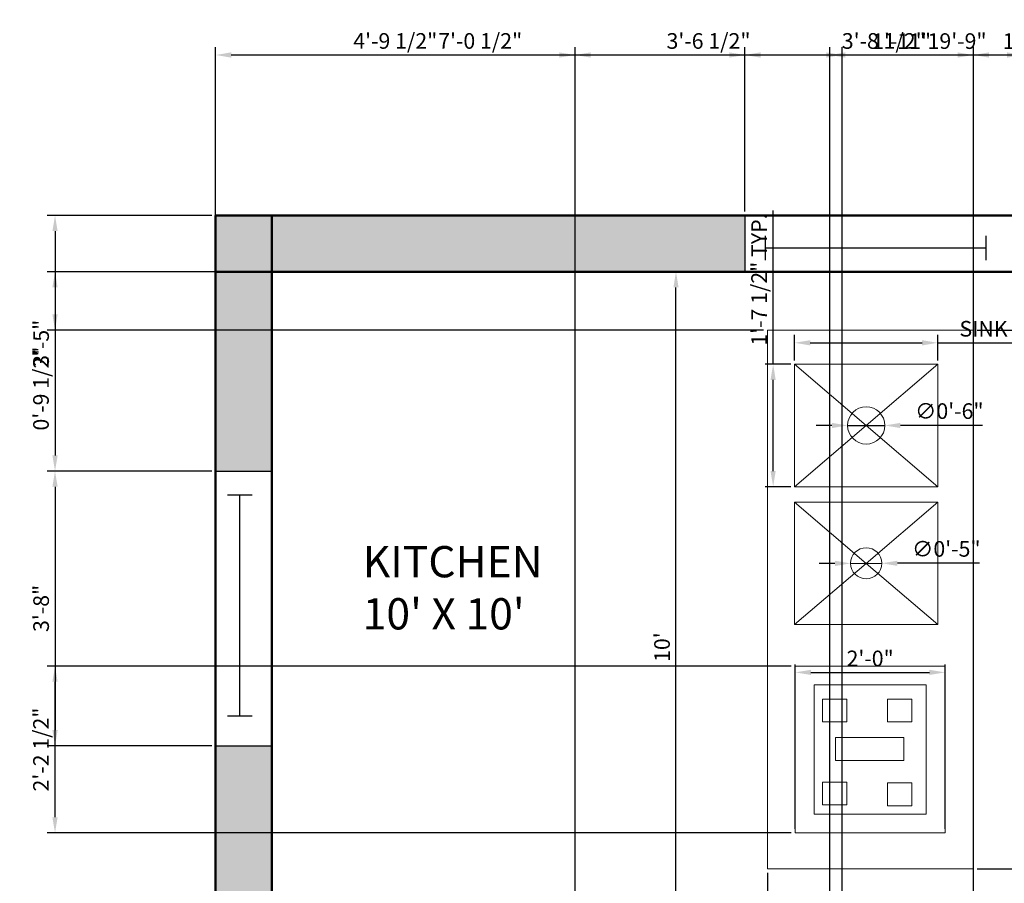
# Model space of a CAD drawing. Units: millimetres. Extents: x 2877 to 3173, y 802 to 1374.
# Tile 4 of 5: x 2877 to 3035, y 1236 to 1374. Entities that reach past the tile are written whole.
import ezdxf

# ---------------------------------------------------------------- set-up
doc = ezdxf.new("R2010")
doc.units = ezdxf.units.MM
for name, color, linetype, lineweight in [('A-AREA-IDEN', 150, 'Continuous', 25), ('A-EQPM', 70, 'Continuous', 18), ('A-FLOR-FIXT', 70, 'Continuous', 18), ('A-WALL-PATT', 3, 'Continuous', 13), ('dimensions', 140, 'Continuous', 18), ('walls', 50, 'Continuous', 50), ('windows', 190, 'Continuous', 25)]:
    doc.layers.add(name, color=color, linetype=linetype, lineweight=lineweight)
doc.styles.get("Standard").update_dxf_attribs({"font": 'arial.ttf'})
doc.dimstyles.new('ISO-25', dxfattribs={"dimtxt": 2.5, "dimasz": 2.5, "dimexe": 1.25, "dimexo": 0.625, "dimtad": 1, "dimdec": 0, "dimlunit": 3, "dimtxsty": 'Standard', "dimcen": 2.5, "dimadec": 0, "dimazin": 0, "dimtfac": 1, "dimtdec": 0, "dimtmove": 0, "dimatfit": 3, "dimfxl": 1, "dimarcsym": 0})

# ---------------------------------------------------------------- blocks, each defined once
blk = doc.blocks.new('*U4')
for p, q in [((0, 4), (0, 0)), ((36, 4), (36, 0)), ((0, 2), (36, 2))]:
    blk.add_line(p, q)
blk = doc.blocks.new('*D11')
at = {"layer": 'Defpoints', "color": 0, "transparency": 16777216}
for p in [(2982.2, 1333.28), (2982.2, 1333.28), (2982.2, 1213.28)]:
    blk.add_point(p, dxfattribs=at)
at = {"layer": 'dimensions', "color": 0, "lineweight": -2, "transparency": 16777216}
for p, q in [((2982.83, 1333.28), (2983.45, 1333.28)), ((2982.2, 1215.78), (2982.2, 1330.78)), ((2982.83, 1213.28), (2983.45, 1213.28))]:
    blk.add_line(p, q, dxfattribs=at)
at = {"layer": 'dimensions', "color": 0, "transparency": 16777216}
for points in [[(2981.79, 1330.78), (2982.62, 1330.78), (2982.2, 1333.28)], [(2981.79, 1215.78), (2982.62, 1215.78), (2982.2, 1213.28)]]:
    blk.add_solid(points, dxfattribs=at)
at = {"layer": 'dimensions', "color": 0, "transparency": 16777216, "insert": (2980.3, 1273.28), "char_height": 2.5, "attachment_point": 5, "rotation": 90}
blk.add_mtext("10'", dxfattribs=at)
blk = doc.blocks.new('SINK-BOWL')
for q in [(0, 19.57), (22.88, 19.57), (0, 0), (22.88, 0)]:
    blk.add_line((11.44, 9.78), q)
blk.add_lwpolyline([(0, 19.57), (22.88, 19.57), (22.88, 0), (0, 0)], close=True)
blk = doc.blocks.new('*D24')
at = {"layer": 'Defpoints', "color": 0, "transparency": 16777216}
for p in [(3024.04, 1321.93), (3001.16, 1318.5), (3024.04, 1318.5)]:
    blk.add_point(p, dxfattribs=at)
at = {"layer": 'dimensions', "color": 0, "lineweight": -2, "transparency": 16777216}
for p, q in [((3001.16, 1319.12), (3001.16, 1323.18)), ((3003.66, 1321.93), (3021.54, 1321.93)), ((3024.04, 1319.12), (3024.04, 1323.18)), ((3024.04, 1321.93), (3054.08, 1321.93))]:
    blk.add_line(p, q, dxfattribs=at)
at = {"layer": 'dimensions', "color": 0, "transparency": 16777216}
for points in [[(3003.66, 1322.35), (3003.66, 1321.51), (3001.16, 1321.93)], [(3021.54, 1322.35), (3021.54, 1321.51), (3024.04, 1321.93)]]:
    blk.add_solid(points, dxfattribs=at)
at = {"layer": 'dimensions', "color": 0, "transparency": 16777216, "insert": (3040.31, 1323.85), "char_height": 2.5, "attachment_point": 5}
blk.add_mtext('SINK 1\'-11" TYP.', dxfattribs=at)
blk = doc.blocks.new('*D25')
at = {"layer": 'Defpoints', "color": 0, "transparency": 16777216}
for p in [(2997.73, 1318.5), (3001.16, 1318.5), (3001.16, 1298.93)]:
    blk.add_point(p, dxfattribs=at)
at = {"layer": 'dimensions', "color": 0, "lineweight": -2, "transparency": 16777216}
for p, q in [((2997.73, 1318.5), (2997.73, 1343.08)), ((3000.53, 1318.5), (2996.48, 1318.5)), ((2997.73, 1301.43), (2997.73, 1316)), ((3000.53, 1298.93), (2996.48, 1298.93))]:
    blk.add_line(p, q, dxfattribs=at)
at = {"layer": 'dimensions', "color": 0, "transparency": 16777216}
for points in [[(2997.31, 1316), (2998.14, 1316), (2997.73, 1318.5)], [(2997.31, 1301.43), (2998.14, 1301.43), (2997.73, 1298.93)]]:
    blk.add_solid(points, dxfattribs=at)
at = {"layer": 'dimensions', "color": 0, "transparency": 16777216, "insert": (2995.81, 1332.04), "char_height": 2.5, "attachment_point": 5, "rotation": 90}
blk.add_mtext('1\'-7 1/2" TYP.', dxfattribs=at)
blk = doc.blocks.new('*D34')
at = {"layer": 'Defpoints', "color": 0, "transparency": 16777216}
for p in [(3145.62, 1367.94), (2908.62, 1342.28), (3145.62, 1342.28)]:
    blk.add_point(p, dxfattribs=at)
at = {"layer": 'dimensions', "color": 0, "lineweight": -2, "transparency": 16777216}
for p, q in [((2908.62, 1342.9), (2908.62, 1369.19)), ((3145.62, 1342.9), (3145.62, 1369.19)), ((2911.12, 1367.94), (3143.12, 1367.94))]:
    blk.add_line(p, q, dxfattribs=at)
at = {"layer": 'dimensions', "color": 0, "transparency": 16777216}
for points in [[(2911.12, 1368.36), (2911.12, 1367.52), (2908.62, 1367.94)], [(3143.12, 1368.36), (3143.12, 1367.52), (3145.62, 1367.94)]]:
    blk.add_solid(points, dxfattribs=at)
at = {"layer": 'dimensions', "color": 0, "transparency": 16777216, "insert": (3027.12, 1369.84), "char_height": 2.5, "attachment_point": 5}
blk.add_mtext('19\'-9"', dxfattribs=at)
blk = doc.blocks.new('*D36')
at = {"layer": 'Defpoints', "color": 0, "transparency": 16777216}
for p in [(2908.62, 1301.43), (2917.62, 1301.43), (2917.62, 803.61)]:
    blk.add_point(p, dxfattribs=at)
at = {"layer": 'dimensions', "color": 0, "lineweight": -2, "transparency": 16777216}
for p, q in [((2908.62, 1300.81), (2908.62, 802.36)), ((2917.62, 1300.81), (2917.62, 802.36)), ((2911.12, 803.61), (2915.12, 803.61))]:
    blk.add_line(p, q, dxfattribs=at)
at = {"layer": 'dimensions', "color": 0, "transparency": 16777216}
for points in [[(2911.12, 804.03), (2911.12, 803.2), (2908.62, 803.61)], [(2915.12, 804.03), (2915.12, 803.2), (2917.62, 803.61)]]:
    blk.add_solid(points, dxfattribs=at)
at = {"layer": 'dimensions', "color": 0, "transparency": 16777216, "insert": (2913.12, 805.52), "char_height": 2.5, "attachment_point": 5}
blk.add_mtext('0\'-9"', dxfattribs=at)
blk = doc.blocks.new('*D44')
at = {"layer": 'Defpoints', "color": 0, "transparency": 16777216}
for p in [(2996.81, 1237.82), (3029.69, 1237.82), (3029.69, 803.61)]:
    blk.add_point(p, dxfattribs=at)
at = {"layer": 'dimensions', "color": 0, "lineweight": -2, "transparency": 16777216}
for p, q in [((2996.81, 1237.19), (2996.81, 802.36)), ((3029.69, 1237.19), (3029.69, 802.36)), ((2999.31, 803.61), (3027.19, 803.61))]:
    blk.add_line(p, q, dxfattribs=at)
at = {"layer": 'dimensions', "color": 0, "transparency": 16777216}
for points in [[(2999.31, 804.03), (2999.31, 803.2), (2996.81, 803.61)], [(3027.19, 804.03), (3027.19, 803.2), (3029.69, 803.61)]]:
    blk.add_solid(points, dxfattribs=at)
at = {"layer": 'dimensions', "color": 0, "transparency": 16777216, "insert": (3013.25, 805.52), "char_height": 2.5, "attachment_point": 5}
blk.add_mtext('2\'-9"', dxfattribs=at)
blk = doc.blocks.new('*D45')
at = {"layer": 'Defpoints', "color": 0, "transparency": 16777216}
for p in [(3029.69, 1323.97), (3171.28, 1323.97), (3029.69, 1237.82)]:
    blk.add_point(p, dxfattribs=at)
at = {"layer": 'dimensions', "color": 0, "lineweight": -2, "transparency": 16777216}
for p, q in [((3030.32, 1323.97), (3172.53, 1323.97)), ((3171.28, 1240.32), (3171.28, 1321.47)), ((3030.32, 1237.82), (3172.53, 1237.82))]:
    blk.add_line(p, q, dxfattribs=at)
at = {"layer": 'dimensions', "color": 0, "transparency": 16777216}
for points in [[(3170.87, 1321.47), (3171.7, 1321.47), (3171.28, 1323.97)], [(3170.87, 1240.32), (3171.7, 1240.32), (3171.28, 1237.82)]]:
    blk.add_solid(points, dxfattribs=at)
at = {"layer": 'dimensions', "color": 0, "transparency": 16777216, "insert": (3169.4, 1280.89), "char_height": 2.5, "attachment_point": 5, "rotation": 90}
blk.add_mtext('7\'-2"', dxfattribs=at)
blk = doc.blocks.new('*D48')
at = {"layer": 'Defpoints', "color": 0, "transparency": 16777216}
for p in [(3029.73, 1367.94), (3006.77, 1144.28), (3029.73, 1144.28)]:
    blk.add_point(p, dxfattribs=at)
at = {"layer": 'dimensions', "color": 0, "lineweight": -2, "transparency": 16777216}
for p, q in [((3006.77, 1144.9), (3006.77, 1369.19)), ((3029.73, 1144.9), (3029.73, 1369.19)), ((3009.27, 1367.94), (3027.23, 1367.94))]:
    blk.add_line(p, q, dxfattribs=at)
at = {"layer": 'dimensions', "color": 0, "transparency": 16777216}
for points in [[(3009.27, 1368.36), (3009.27, 1367.52), (3006.77, 1367.94)], [(3027.23, 1368.36), (3027.23, 1367.52), (3029.73, 1367.94)]]:
    blk.add_solid(points, dxfattribs=at)
at = {"layer": 'dimensions', "color": 0, "transparency": 16777216, "insert": (3018.25, 1369.82), "char_height": 2.5, "attachment_point": 5}
blk.add_mtext('1\'-11"', dxfattribs=at)
blk = doc.blocks.new('*D49')
at = {"layer": 'Defpoints', "color": 0, "transparency": 16777216}
for p in [(3046.62, 1367.94), (3029.73, 1144.28), (3046.62, 1144.28)]:
    blk.add_point(p, dxfattribs=at)
at = {"layer": 'dimensions', "color": 0, "lineweight": -2, "transparency": 16777216}
for p, q in [((3029.73, 1144.9), (3029.73, 1369.19)), ((3046.62, 1144.9), (3046.62, 1369.19)), ((3032.23, 1367.94), (3044.12, 1367.94))]:
    blk.add_line(p, q, dxfattribs=at)
at = {"layer": 'dimensions', "color": 0, "transparency": 16777216}
for points in [[(3032.23, 1368.36), (3032.23, 1367.52), (3029.73, 1367.94)], [(3044.12, 1368.36), (3044.12, 1367.52), (3046.62, 1367.94)]]:
    blk.add_solid(points, dxfattribs=at)
at = {"layer": 'dimensions', "color": 0, "transparency": 16777216, "insert": (3038.18, 1369.84), "char_height": 2.5, "attachment_point": 5}
blk.add_mtext('1\'-5"', dxfattribs=at)
blk = doc.blocks.new('*D50')
at = {"layer": 'Defpoints', "color": 0, "transparency": 16777216}
for p in [(2908.62, 1301.43), (2882.96, 1257.52), (2908.62, 1257.52)]:
    blk.add_point(p, dxfattribs=at)
at = {"layer": 'dimensions', "color": 0, "lineweight": -2, "transparency": 16777216}
for p, q in [((2908, 1301.43), (2881.71, 1301.43)), ((2882.96, 1298.93), (2882.96, 1260.02)), ((2908, 1257.52), (2881.71, 1257.52))]:
    blk.add_line(p, q, dxfattribs=at)
at = {"layer": 'dimensions', "color": 0, "transparency": 16777216}
for points in [[(2882.54, 1298.93), (2883.38, 1298.93), (2882.96, 1301.43)], [(2882.54, 1260.02), (2883.38, 1260.02), (2882.96, 1257.52)]]:
    blk.add_solid(points, dxfattribs=at)
at = {"layer": 'dimensions', "color": 0, "transparency": 16777216, "insert": (2881.06, 1279.47), "char_height": 2.5, "attachment_point": 5, "rotation": 90}
blk.add_mtext('3\'-8"', dxfattribs=at)
blk = doc.blocks.new('*D51')
at = {"layer": 'Defpoints', "color": 0, "transparency": 16777216}
for p in [(2908.62, 1342.28), (2882.96, 1301.43), (2908.62, 1301.43)]:
    blk.add_point(p, dxfattribs=at)
at = {"layer": 'dimensions', "color": 0, "lineweight": -2, "transparency": 16777216}
for p, q in [((2908, 1342.28), (2881.71, 1342.28)), ((2882.96, 1339.78), (2882.96, 1303.93)), ((2908, 1301.43), (2881.71, 1301.43))]:
    blk.add_line(p, q, dxfattribs=at)
at = {"layer": 'dimensions', "color": 0, "transparency": 16777216}
for points in [[(2882.54, 1339.78), (2883.38, 1339.78), (2882.96, 1342.28)], [(2882.54, 1303.93), (2883.38, 1303.93), (2882.96, 1301.43)]]:
    blk.add_solid(points, dxfattribs=at)
at = {"layer": 'dimensions', "color": 0, "transparency": 16777216, "insert": (2881.06, 1321.85), "char_height": 2.5, "attachment_point": 5, "rotation": 90}
blk.add_mtext('3\'-5"', dxfattribs=at)
blk = doc.blocks.new('*D52')
at = {"layer": 'Defpoints', "color": 0, "transparency": 16777216}
for p in [(3037.62, 1367.94), (2993.21, 1342.28), (3037.62, 1342.28)]:
    blk.add_point(p, dxfattribs=at)
at = {"layer": 'dimensions', "color": 0, "lineweight": -2, "transparency": 16777216}
for p, q in [((2993.21, 1342.9), (2993.21, 1369.19)), ((3037.62, 1342.9), (3037.62, 1369.19)), ((2995.71, 1367.94), (3035.12, 1367.94))]:
    blk.add_line(p, q, dxfattribs=at)
at = {"layer": 'dimensions', "color": 0, "transparency": 16777216}
for points in [[(2995.71, 1368.36), (2995.71, 1367.52), (2993.21, 1367.94)], [(3035.12, 1368.36), (3035.12, 1367.52), (3037.62, 1367.94)]]:
    blk.add_solid(points, dxfattribs=at)
at = {"layer": 'dimensions', "color": 0, "transparency": 16777216, "insert": (3015.41, 1369.86), "char_height": 2.5, "attachment_point": 5}
blk.add_mtext('3\'-8 1/2"', dxfattribs=at)
blk = doc.blocks.new('*D53')
at = {"layer": 'Defpoints', "color": 0, "transparency": 16777216}
for p in [(2993.21, 1367.94), (2908.62, 1342.28), (2993.21, 1342.28)]:
    blk.add_point(p, dxfattribs=at)
at = {"layer": 'dimensions', "color": 0, "lineweight": -2, "transparency": 16777216}
for p, q in [((2908.62, 1342.9), (2908.62, 1369.19)), ((2993.21, 1342.9), (2993.21, 1369.19)), ((2911.12, 1367.94), (2990.71, 1367.94))]:
    blk.add_line(p, q, dxfattribs=at)
at = {"layer": 'dimensions', "color": 0, "transparency": 16777216}
for points in [[(2911.12, 1368.36), (2911.12, 1367.52), (2908.62, 1367.94)], [(2990.71, 1368.36), (2990.71, 1367.52), (2993.21, 1367.94)]]:
    blk.add_solid(points, dxfattribs=at)
at = {"layer": 'dimensions', "color": 0, "transparency": 16777216, "insert": (2950.91, 1369.86), "char_height": 2.5, "attachment_point": 5}
blk.add_mtext('7\'-0 1/2"', dxfattribs=at)
blk = doc.blocks.new('*D58')
at = {"layer": 'Defpoints', "color": 0, "transparency": 16777216}
for p in [(2966.07, 1367.94), (2908.62, 943.28), (2966.07, 943.28)]:
    blk.add_point(p, dxfattribs=at)
at = {"layer": 'dimensions', "color": 0, "lineweight": -2, "transparency": 16777216}
for p, q in [((2908.62, 943.9), (2908.62, 1369.19)), ((2966.07, 943.9), (2966.07, 1369.19)), ((2911.12, 1367.94), (2963.57, 1367.94))]:
    blk.add_line(p, q, dxfattribs=at)
at = {"layer": 'dimensions', "color": 0, "transparency": 16777216}
for points in [[(2911.12, 1368.36), (2911.12, 1367.52), (2908.62, 1367.94)], [(2963.57, 1368.36), (2963.57, 1367.52), (2966.07, 1367.94)]]:
    blk.add_solid(points, dxfattribs=at)
at = {"layer": 'dimensions', "color": 0, "transparency": 16777216, "insert": (2937.34, 1369.86), "char_height": 2.5, "attachment_point": 5}
blk.add_mtext('4\'-9 1/2"', dxfattribs=at)
blk = doc.blocks.new('*D59')
at = {"layer": 'Defpoints', "color": 0, "transparency": 16777216}
for p in [(3008.74, 1367.94), (2966.07, 943.28), (3008.74, 943.28)]:
    blk.add_point(p, dxfattribs=at)
at = {"layer": 'dimensions', "color": 0, "lineweight": -2, "transparency": 16777216}
for p, q in [((2966.07, 943.9), (2966.07, 1369.19)), ((3008.74, 943.9), (3008.74, 1369.19)), ((2968.57, 1367.94), (3006.24, 1367.94))]:
    blk.add_line(p, q, dxfattribs=at)
at = {"layer": 'dimensions', "color": 0, "transparency": 16777216}
for points in [[(2968.57, 1368.36), (2968.57, 1367.52), (2966.07, 1367.94)], [(3006.24, 1368.36), (3006.24, 1367.52), (3008.74, 1367.94)]]:
    blk.add_solid(points, dxfattribs=at)
at = {"layer": 'dimensions', "color": 0, "transparency": 16777216, "insert": (2987.4, 1369.86), "char_height": 2.5, "attachment_point": 5}
blk.add_mtext('3\'-6 1/2"', dxfattribs=at)
blk = doc.blocks.new('*D66')
at = {"layer": 'Defpoints', "color": 0, "transparency": 16777216}
for p in [(2917.62, 1257.52), (2996.81, 1237.82), (2996.81, 803.61)]:
    blk.add_point(p, dxfattribs=at)
at = {"layer": 'dimensions', "color": 0, "lineweight": -2, "transparency": 16777216}
for p, q in [((2917.62, 1256.89), (2917.62, 802.36)), ((2996.81, 1237.19), (2996.81, 802.36)), ((2920.12, 803.61), (2994.31, 803.61))]:
    blk.add_line(p, q, dxfattribs=at)
at = {"layer": 'dimensions', "color": 0, "transparency": 16777216}
for points in [[(2920.12, 804.03), (2920.12, 803.2), (2917.62, 803.61)], [(2994.31, 804.03), (2994.31, 803.2), (2996.81, 803.61)]]:
    blk.add_solid(points, dxfattribs=at)
at = {"layer": 'dimensions', "color": 0, "transparency": 16777216, "insert": (2957.22, 805.52), "char_height": 2.5, "attachment_point": 5}
blk.add_mtext('6\'-7"', dxfattribs=at)
blk = doc.blocks.new('*D67')
at = {"layer": 'Defpoints', "color": 0, "transparency": 16777216}
for p in [(2993.21, 1333.28), (2882.96, 1323.97), (2996.81, 1323.97)]:
    blk.add_point(p, dxfattribs=at)
at = {"layer": 'dimensions', "color": 0, "lineweight": -2, "transparency": 16777216}
for p, q in [((2992.58, 1333.28), (2881.71, 1333.28)), ((2882.96, 1330.78), (2882.96, 1326.47)), ((2996.19, 1323.97), (2881.71, 1323.97)), ((2882.96, 1323.97), (2882.96, 1307.75))]:
    blk.add_line(p, q, dxfattribs=at)
at = {"layer": 'dimensions', "color": 0, "transparency": 16777216}
for points in [[(2882.54, 1330.78), (2883.38, 1330.78), (2882.96, 1333.28)], [(2882.54, 1326.47), (2883.38, 1326.47), (2882.96, 1323.97)]]:
    blk.add_solid(points, dxfattribs=at)
at = {"layer": 'dimensions', "color": 0, "transparency": 16777216, "insert": (2881.04, 1314.61), "char_height": 2.5, "attachment_point": 5, "rotation": 90}
blk.add_mtext('0\'-9 1/2"', dxfattribs=at)
blk = doc.blocks.new('*D68')
at = {"layer": 'Defpoints', "color": 0, "transparency": 16777216}
for p in [(3025.21, 1269.24), (3001.26, 1243.58), (3025.21, 1243.58)]:
    blk.add_point(p, dxfattribs=at)
at = {"layer": 'dimensions', "color": 0, "lineweight": -2, "transparency": 16777216}
for p, q in [((3001.26, 1244.21), (3001.26, 1270.49)), ((3025.21, 1244.21), (3025.21, 1270.49)), ((3003.76, 1269.24), (3022.71, 1269.24))]:
    blk.add_line(p, q, dxfattribs=at)
at = {"layer": 'dimensions', "color": 0, "transparency": 16777216}
for points in [[(3003.76, 1269.66), (3003.76, 1268.83), (3001.26, 1269.24)], [(3022.71, 1269.66), (3022.71, 1268.83), (3025.21, 1269.24)]]:
    blk.add_solid(points, dxfattribs=at)
at = {"layer": 'dimensions', "color": 0, "transparency": 16777216, "insert": (3013.23, 1271.15), "char_height": 2.5, "attachment_point": 5}
blk.add_mtext('2\'-0"', dxfattribs=at)
blk = doc.blocks.new('*D69')
at = {"layer": 'Defpoints', "color": 0, "transparency": 16777216}
for p in [(2882.96, 1270.24), (3001.26, 1270.24), (3001.26, 1243.58)]:
    blk.add_point(p, dxfattribs=at)
at = {"layer": 'dimensions', "color": 0, "lineweight": -2, "transparency": 16777216}
for p, q in [((3000.63, 1270.24), (2881.71, 1270.24)), ((2882.96, 1246.08), (2882.96, 1267.74)), ((3000.63, 1243.58), (2881.71, 1243.58))]:
    blk.add_line(p, q, dxfattribs=at)
at = {"layer": 'dimensions', "color": 0, "transparency": 16777216}
for points in [[(2882.54, 1267.74), (2883.38, 1267.74), (2882.96, 1270.24)], [(2882.54, 1246.08), (2883.38, 1246.08), (2882.96, 1243.58)]]:
    blk.add_solid(points, dxfattribs=at)
at = {"layer": 'dimensions', "color": 0, "transparency": 16777216, "insert": (2881.04, 1256.91), "char_height": 2.5, "attachment_point": 5, "rotation": 90}
blk.add_mtext('2\'-2 1/2"', dxfattribs=at)
blk = doc.blocks.new('*D70')
at = {"layer": 'Defpoints', "color": 0, "transparency": 16777216}
for p in [(3010.11, 1286.67), (3015.09, 1286.68)]:
    blk.add_point(p, dxfattribs=at)
at = {"layer": 'dimensions', "color": 0, "lineweight": -2, "transparency": 16777216}
for p, q in [((3007.61, 1286.67), (3005.11, 1286.67)), ((3010.11, 1286.67), (3015.09, 1286.68)), ((3030.71, 1286.7), (3017.59, 1286.68))]:
    blk.add_line(p, q, dxfattribs=at)
at = {"layer": 'dimensions', "color": 0, "transparency": 16777216}
for points in [[(3007.6, 1287.09), (3007.61, 1286.25), (3010.11, 1286.67)], [(3017.59, 1287.1), (3017.59, 1286.27), (3015.09, 1286.68)]]:
    blk.add_solid(points, dxfattribs=at)
at = {"layer": 'dimensions', "color": 0, "transparency": 16777216, "insert": (3025.4, 1288.66), "char_height": 2.5, "attachment_point": 5, "rotation": 0.0643}
blk.add_mtext('∅0\'-5"', dxfattribs=at)
blk = doc.blocks.new('*D71')
at = {"layer": 'Defpoints', "color": 0, "transparency": 16777216}
for p in [(3009.62, 1308.72), (3015.57, 1308.72)]:
    blk.add_point(p, dxfattribs=at)
at = {"layer": 'dimensions', "color": 0, "lineweight": -2, "transparency": 16777216}
for p, q in [((3007.12, 1308.72), (3004.62, 1308.72)), ((3009.62, 1308.72), (3015.57, 1308.72)), ((3031.19, 1308.72), (3018.07, 1308.72))]:
    blk.add_line(p, q, dxfattribs=at)
at = {"layer": 'dimensions', "color": 0, "transparency": 16777216}
for points in [[(3007.12, 1309.13), (3007.12, 1308.3), (3009.62, 1308.72)], [(3018.07, 1309.13), (3018.07, 1308.3), (3015.57, 1308.72)]]:
    blk.add_solid(points, dxfattribs=at)
at = {"layer": 'dimensions', "color": 0, "transparency": 16777216, "insert": (3025.88, 1310.69), "char_height": 2.5, "attachment_point": 5, "rotation": 0.0048}
blk.add_mtext('∅0\'-6"', dxfattribs=at)

msp = doc.modelspace()

# ---------------------------------------------------------------- hatches: boundary and pattern name
at = {"layer": 'A-WALL-PATT'}
h = msp.add_hatch(color=256, dxfattribs=at)
h.dxf.hatch_style = 1
h.paths.add_polyline_path([(3046.62, 1333.28), (3037.62, 1333.28), (3037.62, 1273.28), (3046.62, 1273.28)])
h.paths.add_polyline_path([(3046.62, 1273.28), (3037.62, 1273.28), (3037.62, 1264.28), (3046.62, 1264.28)])
h.paths.add_polyline_path([(3046.62, 1264.28), (3037.62, 1264.28), (3037.62, 1204.28), (3046.62, 1204.28)])
h.paths.add_polyline_path([(3136.62, 1273.28), (3099.39, 1273.28), (3099.39, 1264.28), (3136.62, 1264.28)])
h.paths.add_polyline_path([(3145.62, 1273.28), (3136.62, 1273.28), (3136.62, 1264.28), (3145.62, 1264.28)])
h.paths.add_polyline_path([(3145.62, 1264.28), (3136.62, 1264.28), (3136.62, 1198.76), (3145.62, 1198.76)])
h.paths.add_polyline_path([(3145.62, 1333.28), (3136.62, 1333.28), (3136.62, 1273.28), (3145.62, 1273.28)])
h.paths.add_polyline_path([(3145.62, 1342.28), (3136.62, 1342.28), (3136.62, 1333.28), (3145.62, 1333.28)])
h.paths.add_polyline_path([(3136.62, 1342.28), (3046.62, 1342.28), (3046.62, 1333.28), (3136.62, 1333.28)])
h.paths.add_polyline_path([(3046.62, 1342.28), (3037.62, 1342.28), (3037.62, 1333.28), (3046.62, 1333.28)])
h.paths.add_polyline_path([(2917.62, 1333.28), (2908.62, 1333.28), (2908.62, 1301.43), (2917.62, 1301.43)])
h.paths.add_polyline_path([(2917.62, 1257.52), (2908.62, 1257.52), (2908.62, 1213.28), (2917.62, 1213.28)])
h.paths.add_polyline_path([(2989.62, 1213.28), (2917.62, 1213.28), (2917.62, 1204.28), (2989.62, 1204.28)])
h.paths.add_polyline_path([(2998.62, 1213.28), (2989.62, 1213.28), (2989.62, 1204.28), (2998.62, 1204.28)])
h.paths.add_polyline_path([(2998.62, 1204.28), (2989.62, 1204.28), (2989.62, 1144.28), (2998.62, 1144.28)])
h.paths.add_polyline_path([(2998.62, 1144.28), (2989.62, 1144.28), (2989.62, 1135.28), (2998.62, 1135.28)])
h.paths.add_polyline_path([(2989.62, 1144.28), (2977.25, 1144.28), (2977.25, 1137.64), (2977.25, 1135.28), (2989.62, 1135.28)])
h.paths.add_polyline_path([(3006.77, 1141.79), (3006.77, 1144.28), (2998.62, 1144.28), (2998.62, 1135.28), (3007.71, 1135.28, -0.072018)])
h.paths.add_polyline_path([(3046.62, 1135.28), (3037.62, 1135.28), (3037.62, 1012.28), (3046.62, 1012.28)])
h.paths.add_polyline_path([(3046.62, 1144.28), (3037.62, 1144.28), (3037.62, 1135.28), (3046.62, 1135.28)])
h.paths.add_polyline_path([(3037.62, 1144.28), (3029.73, 1144.28), (3029.73, 1141.79), (3029.73, 1135.28), (3037.62, 1135.28)])
h.paths.add_polyline_path([(3145.62, 1158.87), (3136.62, 1158.87), (3136.62, 1012.28), (3145.62, 1012.28)])
h.paths.add_polyline_path([(3145.62, 1003.28), (3136.62, 1003.28), (3136.62, 838.28), (3145.62, 838.28)])
h.paths.add_polyline_path([(3145.62, 1012.28), (3136.62, 1012.28), (3136.62, 1003.28), (3145.62, 1003.28)])
h.paths.add_polyline_path([(3136.62, 1012.28), (3109.83, 1012.28), (3109.83, 1006.01), (3109.83, 1003.28), (3136.62, 1003.28)])
h.paths.add_polyline_path([(3073.41, 1012.28), (3046.62, 1012.28), (3046.62, 1003.28), (3073.41, 1003.28), (3073.41, 1006.01)])
h.paths.add_polyline_path([(3046.62, 1012.28), (3037.62, 1012.28), (3037.62, 1003.28), (3046.62, 1003.28)])
h.paths.add_polyline_path([(3046.62, 1003.28), (3037.62, 1003.28), (3037.62, 943.28), (3046.62, 943.28)])
h.paths.add_polyline_path([(3136.62, 838.28), (2917.62, 838.28), (2917.62, 829.28), (3136.62, 829.28)])
h.paths.add_polyline_path([(3145.62, 838.28), (3136.62, 838.28), (3136.62, 829.28), (3145.62, 829.28)])
h.paths.add_polyline_path([(2917.62, 934.28), (2908.62, 934.28), (2908.62, 838.28), (2917.62, 838.28)])
h.paths.add_polyline_path([(2917.62, 838.28), (2908.62, 838.28), (2908.62, 829.28), (2917.62, 829.28)])
h.paths.add_polyline_path([(2917.62, 943.28), (2908.62, 943.28), (2908.62, 934.28), (2917.62, 934.28)])
h.paths.add_polyline_path([(2966.07, 943.28), (2917.62, 943.28), (2917.62, 934.28), (2966.07, 934.28)])
h.paths.add_polyline_path([(3046.62, 943.28), (3037.62, 943.28), (3037.62, 934.28), (3046.62, 934.28)])
h.paths.add_polyline_path([(3037.62, 943.28), (3008.74, 943.28), (3008.74, 934.28), (3037.62, 934.28)])
h = msp.add_hatch(color=256, dxfattribs=at)
h.dxf.hatch_style = 1
h.paths.add_polyline_path([(2993.21, 1342.28), (2917.62, 1342.28), (2917.62, 1333.28), (2993.21, 1333.28)])
h.paths.add_polyline_path([(2917.62, 1342.28), (2908.62, 1342.28), (2908.62, 1333.28), (2917.62, 1333.28)])

# ---------------------------------------------------------------- linework, layer by layer
at = {"layer": 'A-EQPM'}
for points in [[(3025.21, 1270.24), (3001.26, 1270.24), (3001.26, 1243.58), (3025.21, 1243.58)], [(3022.21, 1267.24), (3004.26, 1267.24), (3004.26, 1246.58), (3022.21, 1246.58)], [(3005.62, 1264.98), (3009.52, 1264.98), (3009.52, 1261.32), (3005.62, 1261.32)], [(3016.01, 1264.98), (3019.91, 1264.98), (3019.91, 1261.32), (3016.01, 1261.32)], [(3007.69, 1258.85), (3018.61, 1258.85), (3018.61, 1255.17), (3007.69, 1255.17)], [(3005.62, 1251.71), (3009.52, 1251.71), (3009.52, 1248.05), (3005.62, 1248.05)], [(3016.01, 1251.59), (3019.91, 1251.59), (3019.91, 1247.93), (3016.01, 1247.93)]]:
    msp.add_lwpolyline(points, close=True, dxfattribs=at)
at = {"layer": 'A-FLOR-FIXT'}
msp.add_lwpolyline([(3029.69, 1323.97), (2996.81, 1323.97), (2996.81, 1237.82), (3029.69, 1237.82)], close=True, dxfattribs=at)
for centre, radius in [((3012.6, 1308.72), 2.98), ((3012.6, 1286.68), 2.49)]:
    msp.add_circle(centre, radius, dxfattribs=at)
at = {"layer": 'walls'}
for p, q in [((2908.62, 1342.28), (2908.62, 829.28)), ((2908.62, 1342.28), (3145.62, 1342.28)), ((2917.62, 1342.28), (2917.62, 829.28)), ((2908.62, 1333.28), (3145.62, 1333.28))]:
    msp.add_line(p, q, dxfattribs=at)
at = {"layer": 'windows'}
for p, q in [((2993.21, 1342.28), (2993.21, 1333.28)), ((2908.62, 1301.43), (2917.62, 1301.43)), ((2908.62, 1257.52), (2917.62, 1257.52))]:
    msp.add_line(p, q, dxfattribs=at)

# ---------------------------------------------------------------- block references
at = {"layer": 'A-FLOR-FIXT'}
for p in [(3001.16, 1298.93), (3001.16, 1276.89)]:
    msp.add_blockref('SINK-BOWL', p, dxfattribs=at)
at = {"layer": 'windows', "xscale": 0.9804508946843826, "yscale": 0.9804508946843826, "zscale": 0.9804508946843826}
msp.add_blockref('*U4', (2996.43, 1335.13), dxfattribs=at)
at = {"layer": 'windows', "xscale": 0.9804508946843826, "yscale": 0.9804508946843826, "zscale": 0.9804508946843826, "rotation": 90}
msp.add_blockref('*U4', (2914.46, 1262.32), dxfattribs=at)

# ---------------------------------------------------------------- texts
at = {"layer": 'A-AREA-IDEN', "insert": (2932.13, 1289.44), "char_height": 5, "attachment_point": 1}
msp.add_mtext_dynamic_manual_height_columns("KITCHEN\\P10' X 10'", width=47.7685, gutter_width=12.5, heights=[0], dxfattribs=at)

# ---------------------------------------------------------------- dimensions: what is measured, and where the dimension line sits
at = {"layer": 'dimensions'}
for base, p1, p2, picture, middle in [((2993.21, 1367.94), (2908.62, 1342.28), (2993.21, 1342.28), '*D53', (2950.91, 1369.86)), ((2966.066, 1367.9388), (2908.6223, 943.2763), (2966.066, 943.2763), '*D58', (2937.3441, 1369.8564)), ((3008.74, 1367.94), (2966.07, 943.28), (3008.74, 943.28), '*D59', (2987.4, 1369.86)), ((3037.62, 1367.94), (2993.21, 1342.28), (3037.62, 1342.28), '*D52', (3015.41, 1369.86)), ((3145.62, 1367.94), (2908.62, 1342.28), (3145.62, 1342.28), '*D34', (3027.12, 1369.84)), ((3029.73, 1367.94), (3006.77, 1144.28), (3029.73, 1144.28), '*D48', (3018.25, 1369.82)), ((3046.62, 1367.94), (3029.73, 1144.28), (3046.62, 1144.28), '*D49', (3038.18, 1369.84)), ((2917.62, 803.61), (2908.62, 1301.43), (2917.62, 1301.43), '*D36', (2913.12, 805.52)), ((3025.2068, 1269.2436), (3001.2575, 1243.5811), (3025.2068, 1243.5811), '*D68', (3013.2321, 1271.1451)), ((2996.81, 803.61), (2917.62, 1257.52), (2996.81, 1237.82), '*D66', (2957.22, 805.52)), ((3029.69, 803.61), (2996.81, 1237.82), (3029.69, 1237.82), '*D44', (3013.25, 805.52))]:
    dim = msp.add_linear_dim(base=base, p1=p1, p2=p2, dimstyle='ISO-25', override={"dimdec": 1, "dimlfac": 1, "dimrnd": 0, "dimzin": 1, "dimdsep": 46, "dimlunit": 4, "dimfrac": 2}, dxfattribs=at)
    dim.commit()
    dim.dimension.update_dxf_attribs({"geometry": picture, "text_midpoint": middle})
for base, p1, p2, override, picture, middle in [((2882.9598, 1301.4319), (2908.6223, 1342.2763), (2908.6223, 1301.4319), {"dimdec": 1, "dimlfac": 1, "dimrnd": 0, "dimzin": 1, "dimdsep": 46, "dimlunit": 4, "dimfrac": 2}, '*D51', (2881.0575, 1321.8541)), ((2882.96, 1323.97), (2993.21, 1333.28), (2996.81, 1323.97), {"dimdec": 1, "dimlfac": 1, "dimrnd": 0, "dimzin": 1, "dimdsep": 46, "dimlunit": 4, "dimfrac": 2}, '*D67', (2881.04, 1314.61)), ((2982.2, 1333.28), (2982.2, 1213.28), (2982.2, 1333.28), {"dimclrd": 0, "dimclre": 0, "dimclrt": 0}, '*D11', (2980.3, 1273.28)), ((3171.2848, 1323.9689), (3029.6924, 1237.8157), (3029.6924, 1323.9689), {"dimdec": 1, "dimlfac": 1, "dimrnd": 0, "dimzin": 1, "dimdsep": 46, "dimlunit": 4, "dimfrac": 2}, '*D45', (3169.4047, 1280.8923)), ((2882.96, 1257.52), (2908.62, 1301.43), (2908.62, 1257.52), {"dimdec": 1, "dimlfac": 1, "dimrnd": 0, "dimzin": 1, "dimdsep": 46, "dimlunit": 4, "dimfrac": 2}, '*D50', (2881.06, 1279.47)), ((2882.96, 1270.24), (3001.26, 1243.58), (3001.26, 1270.24), {"dimdec": 1, "dimlfac": 1, "dimrnd": 0, "dimzin": 1, "dimdsep": 46, "dimlunit": 4, "dimfrac": 2}, '*D69', (2881.04, 1256.91))]:
    dim = msp.add_linear_dim(base=base, p1=p1, p2=p2, angle=90, dimstyle='ISO-25', override=override, dxfattribs=at)
    dim.commit()
    dim.dimension.update_dxf_attribs({"geometry": picture, "text_midpoint": middle})
dim = msp.add_linear_dim(base=(2997.73, 1318.5), p1=(3001.16, 1298.93), p2=(3001.16, 1318.5), angle=90, text='<> TYP.', dimstyle='ISO-25', override={"dimdec": 1, "dimlfac": 1, "dimrnd": 0, "dimzin": 1, "dimdsep": 46, "dimlunit": 4, "dimfrac": 2}, dxfattribs=at)
dim.commit()
dim.dimension.update_dxf_attribs({"geometry": '*D25', "text_midpoint": (2995.81, 1332.04)})
dim = msp.add_linear_dim(base=(3024.04, 1321.93), p1=(3001.16, 1318.5), p2=(3024.04, 1318.5), text='SINK <> TYP.', dimstyle='ISO-25', override={"dimdec": 1, "dimlfac": 1, "dimrnd": 0, "dimzin": 1, "dimdsep": 46, "dimlunit": 4, "dimfrac": 2}, dxfattribs=at)
dim.commit()
dim.dimension.update_dxf_attribs({"geometry": '*D24', "text_midpoint": (3040.31, 1323.85)})
dim = msp.add_diameter_dim_2p(p1=(3009.6242, 1308.7165), p2=(3015.575, 1308.717), dimstyle='ISO-25', override={"dimdec": 1, "dimlfac": 1, "dimrnd": 0, "dimzin": 1, "dimdsep": 46, "dimlunit": 4, "dimfrac": 2}, dxfattribs=at)
dim.commit()
dim.dimension.update_dxf_attribs({"geometry": '*D71', "text_midpoint": (3025.8828, 1308.7179)})
dim = msp.add_diameter_dim_2p(p1=(3010.11, 1286.67), p2=(3015.09, 1286.68), dimstyle='ISO-25', override={"dimdec": 1, "dimlfac": 1, "dimrnd": 0, "dimzin": 1, "dimdsep": 46, "dimlunit": 4, "dimfrac": 2}, dxfattribs=at)
dim.commit()
dim.dimension.update_dxf_attribs({"geometry": '*D70', "text_midpoint": (3025.4, 1286.69), "dimtype": 163})

doc.saveas('drawing.dxf')
